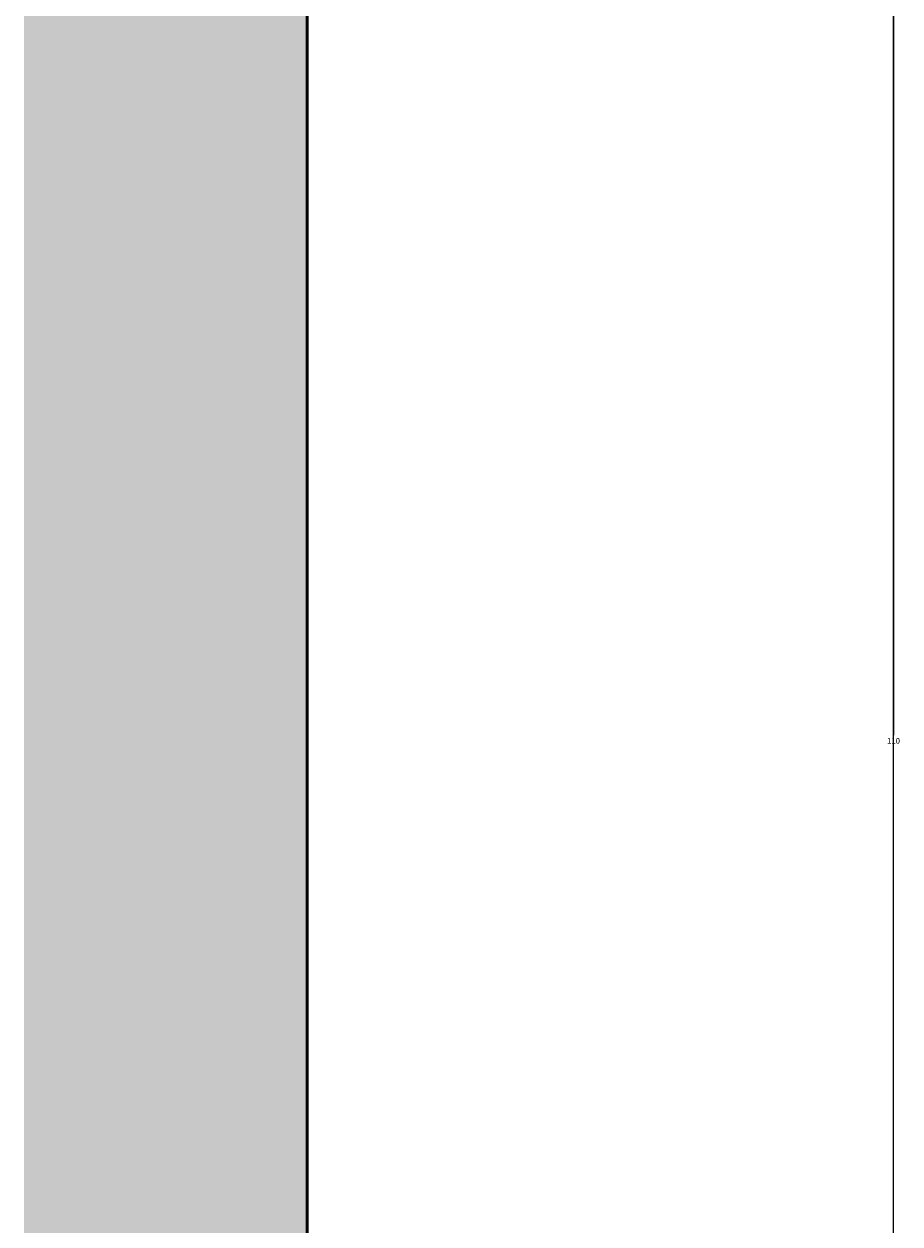
# Model space of a CAD drawing. Units: inches. Extents: x 2231 to 2461, y 2045 to 2455.
# Tile 32 of 95: x 2433 to 2461, y 2112 to 2151. Entities that reach past the tile are written whole.
import ezdxf

# ---------------------------------------------------------------- set-up
doc = ezdxf.new("R2010")
doc.units = ezdxf.units.IN
doc.layers.add('A-ANNO-DIMS', color=2, linetype='Continuous', lineweight=18)
doc.layers.add('A-WALL', color=7, linetype='Continuous', lineweight=50)
doc.layers.add('A-WALL-PATT', color=18, linetype='Continuous', lineweight=13, true_color=0x000000)
doc.styles.get("Standard").update_dxf_attribs({"font": 'arial.ttf'})
doc.dimstyles.get("Standard").update_dxf_attribs({"dimtxt": 0.18, "dimasz": 0.18, "dimexe": 0.18, "dimexo": 0.0625, "dimgap": 0.09, "dimtad": 0, "dimtih": 1, "dimtoh": 1, "dimdec": 4, "dimzin": 0, "dimdsep": 46, "dimtxsty": 'Standard', "dimcen": 0.09, "dimadec": 0, "dimazin": 0, "dimtfac": 1, "dimtdec": 4, "dimtofl": 0, "dimtmove": 0, "dimatfit": 3, "dimfxl": 1, "dimtolj": 1, "dimtzin": 0, "dimarcsym": 0})

# ---------------------------------------------------------------- blocks, each defined once
blk = doc.blocks.new('*D34')
at = {"layer": 'A-ANNO-DIMS', "color": 0, "lineweight": -2, "transparency": 16777216}
for p, q in [((2441.856, 2435.833), (2460.606, 2435.833)), ((2460.426, 2435.653), (2460.426, 2250.015)), ((2460.426, 2064.013), (2460.426, 2249.651)), ((2441.856, 2063.833), (2460.606, 2063.833))]:
    blk.add_line(p, q, dxfattribs=at)
at = {"layer": 'A-ANNO-DIMS', "color": 0, "transparency": 16777216}
for points in [[(2460.396, 2435.653), (2460.456, 2435.653), (2460.426, 2435.833)], [(2460.396, 2064.013), (2460.456, 2064.013), (2460.426, 2063.833)]]:
    blk.add_solid(points, dxfattribs=at)
at = {"layer": 'Defpoints', "color": 0, "transparency": 16777216}
for p in [(2441.794, 2435.833), (2460.426, 2435.833), (2441.794, 2063.833)]:
    blk.add_point(p, dxfattribs=at)
at = {"layer": 'A-ANNO-DIMS', "color": 0, "transparency": 16777216, "insert": (2460.426, 2249.833), "char_height": 0.18, "attachment_point": 5}
blk.add_mtext('\\A1;372', dxfattribs=at)
blk = doc.blocks.new('*D41')
at = {"layer": 'A-ANNO-DIMS', "color": 0, "lineweight": -2, "transparency": 16777216}
for p, q in [((2432.856, 2182.833), (2460.606, 2182.833)), ((2460.426, 2182.653), (2460.426, 2128.015)), ((2460.426, 2073.013), (2460.426, 2127.651)), ((2432.856, 2072.833), (2460.606, 2072.833))]:
    blk.add_line(p, q, dxfattribs=at)
at = {"layer": 'A-ANNO-DIMS', "color": 0, "transparency": 16777216}
for points in [[(2460.396, 2182.653), (2460.456, 2182.653), (2460.426, 2182.833)], [(2460.396, 2073.013), (2460.456, 2073.013), (2460.426, 2072.833)]]:
    blk.add_solid(points, dxfattribs=at)
at = {"layer": 'Defpoints', "color": 0, "transparency": 16777216}
for p in [(2432.794, 2182.833), (2460.426, 2182.833), (2432.794, 2072.833)]:
    blk.add_point(p, dxfattribs=at)
at = {"layer": 'A-ANNO-DIMS', "color": 0, "transparency": 16777216, "insert": (2460.426, 2127.833), "char_height": 0.18, "attachment_point": 5}
blk.add_mtext('\\A1;110', dxfattribs=at)

msp = doc.modelspace()

# ---------------------------------------------------------------- hatches: boundary and pattern name
at = {"layer": 'A-WALL-PATT'}
h = msp.add_hatch(color=256, dxfattribs=at)
h.dxf.hatch_style = 1
h.paths.add_polyline_path([(2441.7935, 2269.1535), (2432.7935, 2269.1535), (2432.7935, 2186.8328), (2396.7935, 2186.8328), (2396.7935, 2286.8328), (2394.7935, 2286.8328), (2394.7935, 2186.8328), (2334.7935, 2186.8328), (2334.7935, 2182.8328), (2432.7935, 2182.8328), (2432.7935, 2072.8328), (2416.6639, 2072.8328), (2416.6639, 2063.8328), (2441.7935, 2063.8328)])
h.paths.add_polyline_path([(2368.6639, 2072.8328), (2367.04, 2072.8328), (2330.7942, 2072.8328), (2330.7397, 2063.8328), (2368.6639, 2063.8328)])
h.paths.add_polyline_path([(2300.7392, 2068.3328), (2300.7392, 2072.8328), (2298.7935, 2072.8328), (2294.7935, 2072.8328), (2258.7935, 2072.8328), (2258.7935, 2120.8328), (2294.7935, 2120.8328), (2298.7935, 2120.8328), (2298.7935, 2128.8328), (2294.7935, 2128.8328), (2294.7935, 2124.8328), (2258.7935, 2124.8328), (2258.7935, 2182.8328), (2294.7935, 2182.8328), (2294.7935, 2174.8328), (2298.7935, 2174.8328), (2298.7935, 2182.8328), (2304.7935, 2182.8328), (2304.7935, 2186.8328), (2258.7935, 2186.8328), (2258.7935, 2221.999), (2249.7935, 2221.999), (2249.7935, 2063.8328), (2300.7392, 2063.8328)])
h.paths.add_polyline_path([(2391.9338, 2435.8328), (2333.82, 2435.8328), (2333.82, 2426.8328), (2368.7935, 2426.8328), (2368.7935, 2374.9508), (2368.7935, 2370.8328), (2372.3935, 2370.8328), (2372.7935, 2370.8328), (2372.7935, 2426.8328), (2391.9338, 2426.8328)])
h.paths.add_polyline_path([(2441.7935, 2435.8328), (2415.9338, 2435.8328), (2415.9338, 2426.8328), (2432.7935, 2426.8328), (2432.7935, 2334.8328), (2372.7935, 2334.8328), (2372.7935, 2346.8328), (2368.7935, 2346.8328), (2368.7935, 2306.8328), (2360.7935, 2306.8328), (2360.7935, 2302.8328), (2368.7935, 2302.8328), (2372.7935, 2302.8328), (2372.7935, 2330.8328), (2432.7935, 2330.8328), (2432.7935, 2317.1535), (2441.7935, 2317.1535)])
h.paths.add_polyline_path([(2285.82, 2435.8328), (2249.7935, 2435.8328), (2249.7935, 2269.999), (2258.7935, 2269.999), (2258.7935, 2302.8328), (2318.8168, 2302.8328), (2330.7935, 2302.8328), (2330.7935, 2306.8328), (2258.7935, 2306.8328), (2258.7935, 2426.8328), (2285.82, 2426.8328)])

# ---------------------------------------------------------------- linework, layer by layer
at = {"layer": 'A-WALL'}
msp.add_lwpolyline([(2300.7392, 2063.8328), (2249.7935, 2063.8328), (2249.7935, 2435.8328), (2441.7935, 2435.8328), (2441.7935, 2063.8328), (2330.7397, 2063.8328)], dxfattribs=at)

# ---------------------------------------------------------------- dimensions: what is measured, and where the dimension line sits
at = {"layer": 'A-ANNO-DIMS'}
for base, p1, p2, picture, middle in [((2460.426, 2435.8328), (2441.7935, 2063.8328), (2441.7935, 2435.8328), '*D34', (2460.426, 2249.8328)), ((2460.426, 2182.8328), (2432.7935, 2072.8328), (2432.7935, 2182.8328), '*D41', (2460.426, 2127.8328))]:
    dim = msp.add_linear_dim(base=base, p1=p1, p2=p2, angle=90, dimstyle='Standard', override={"dimdec": 0, "dimlfac": 1, "dimrnd": 0, "dimzin": 0, "dimdsep": 46, "dimlunit": 2}, dxfattribs=at)
    dim.commit()
    dim.dimension.update_dxf_attribs({"geometry": picture, "text_midpoint": middle})

doc.saveas('drawing.dxf')
